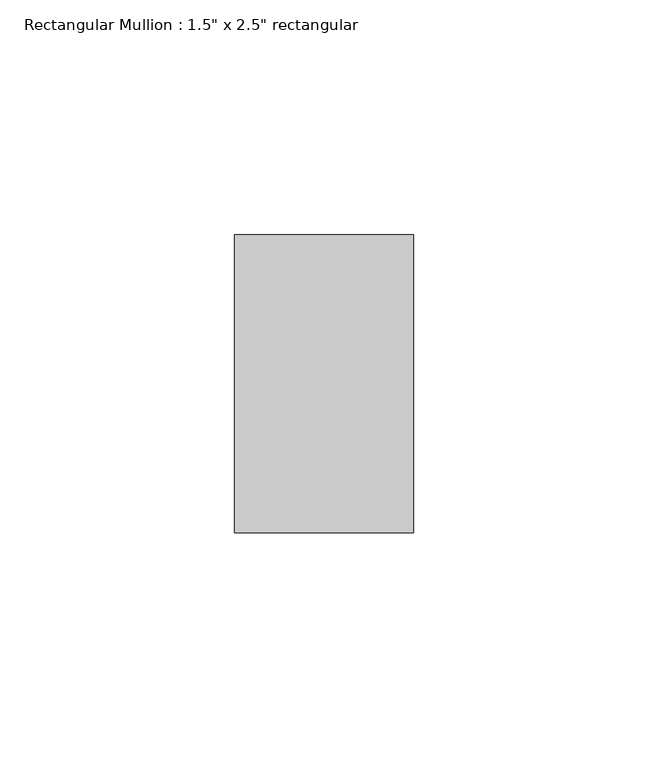
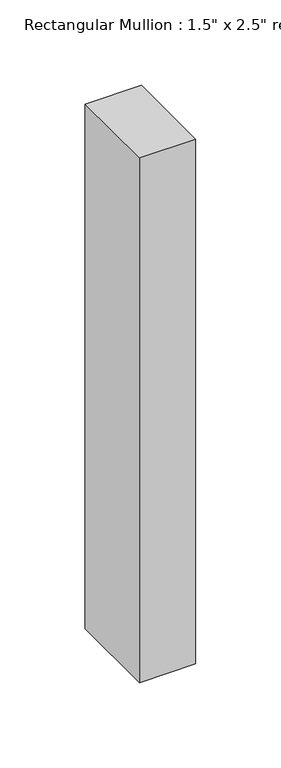
"""IFC4 building model written with IfcOpenShell, lengths in millimetres: member geometry."""

from ifc_helpers import new_model, si_unit, frame, origin, place, context, project, spatial, polyline, outline, extrude, source, transform, mapped, element, save


def member_bd75388b(model_context):
    return source(origin(), model_context, "Body", "SweptSolid", [
        extrude(outline(polyline([(19.05, 31.75), (19.05, -31.75), (-19.05, -31.75), (-19.05, 31.75), (19.05, 31.75)])), frame((0.0, 0.0, -375.1532928), z_axis=(0.0, 0.0, 1.0), x_axis=(1.0, 0.0, 0.0)), (0.0, 0.0, 1.0), 375.1532928),
    ])


if __name__ == "__main__":
    model = new_model("IFC4")
    model_context = context("Model", 3, world=origin())
    ifc_project = project(units=[si_unit("LENGTHUNIT", "METRE", prefix="MILLI")], contexts=[model_context])
    site = spatial("IfcSite", under=ifc_project)
    building = spatial("IfcBuilding", under=site)
    placement = place(None, origin())
    member_shape = member_bd75388b(model_context)
    element("IfcMember", 1, ObjectType="Rectangular Mullion : 1.5\" x 2.5\" rectangular", at=placement, inside=building, context=model_context, shape_type="MappedRepresentation", body=[
        mapped(member_shape, transform((0.0, 0.0, 0.0), x_axis=(1.0, 0.0, 0.0), y_axis=(0.0, 1.0, 0.0), z_axis=(0.0, 0.0, 1.0))),
    ])
    save(model, "model.ifc")

# Revit data of these elements
# Type "Rectangular Mullion : 1.5\" x 2.5\" rectangular"
#   built-in parameter 1007304 = 0.208333 (stored number, unit not read)
#   built-in parameter 1007301 = 0.0625 (stored number, unit not read)
#   built-in parameter 1007300 = 0.0625 (stored number, unit not read)
# Element 1 (IfcMember, "Rectangular Mullion : 1.5\" x 2.5\" rectangular")
#   Materials on its faces: "Aluminum"
# Materials
#   "Aluminum": class "Metal", colour RGB 247 247 247, transparency 0, Description = "Aluminum 6061", Cost = 0
